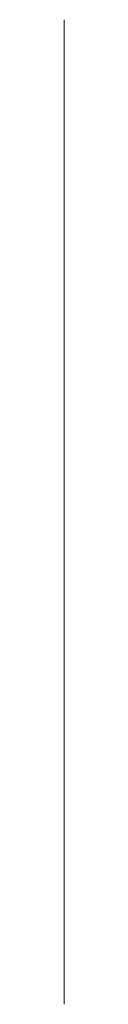
# Model space of a CAD drawing. Units: millimetres. Extents: x 2286.1 to 2286.1, y 931.1 to 954.1.
import ezdxf

# ---------------------------------------------------------------- set-up
doc = ezdxf.new("R2010")
doc.units = ezdxf.units.MM
doc.layers.add('M-CONS', color=8, linetype='Continuous', lineweight=13)

msp = doc.modelspace()

# ---------------------------------------------------------------- linework, layer by layer
at = {"layer": 'M-CONS'}
msp.add_polyline3d([(2286.103, 954.073, 43.575), (2286.103, 931.073, 8), (2286.103, 954.073, 8)], close=True, dxfattribs=at)

doc.saveas('drawing.dxf')
